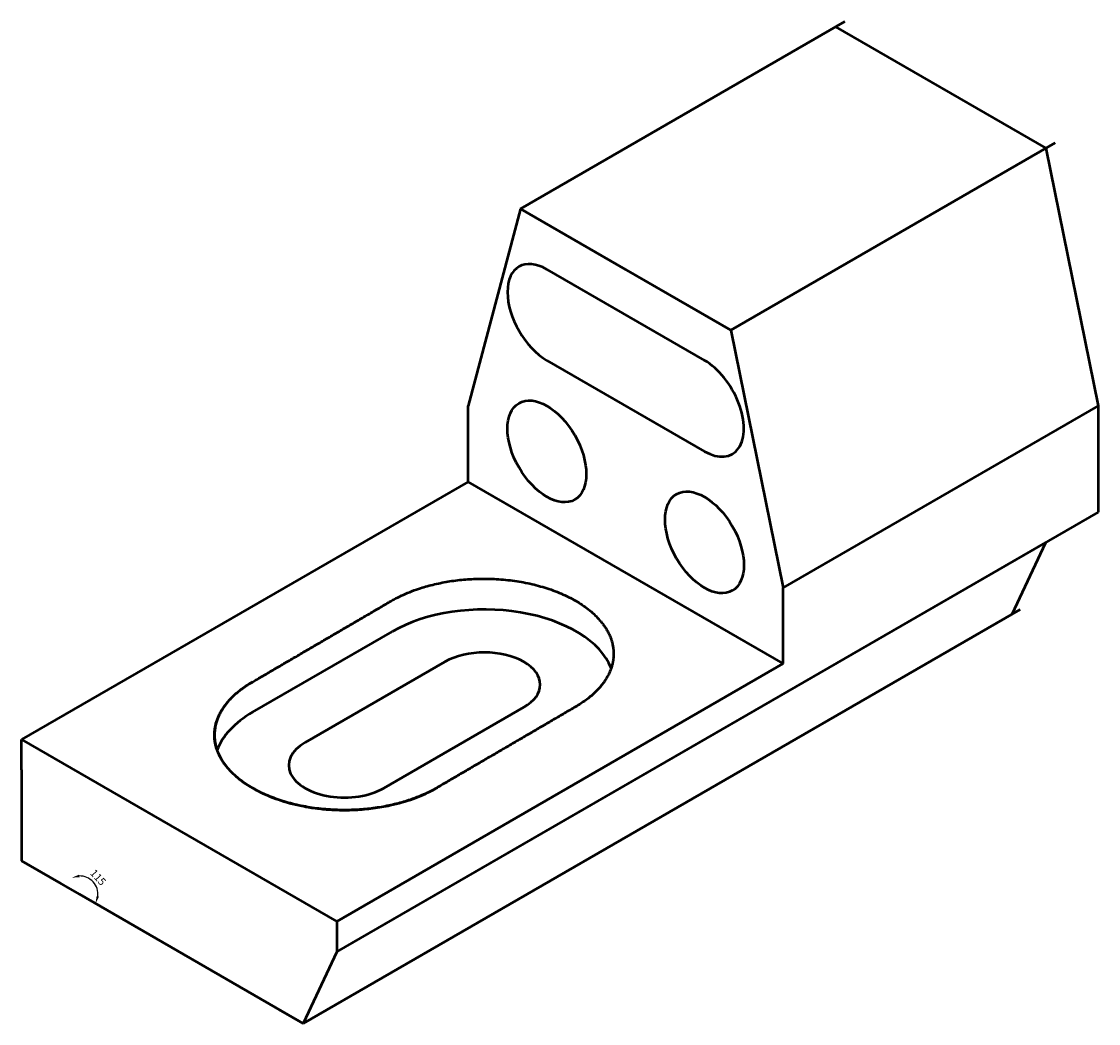
# Model space of a CAD drawing. Units: millimetres. Extents: x 15418 to 15773, y 14576 to 14907.
import ezdxf

# ---------------------------------------------------------------- set-up
doc = ezdxf.new("R2010")
doc.units = ezdxf.units.MM
doc.layers.add('M-DIMS', color=2, linetype='Continuous', lineweight=25)
doc.layers.add('M-OUTL', color=7, linetype='Continuous', lineweight=50)
doc.styles.get("Standard").update_dxf_attribs({"font": 'arial.ttf'})
doc.dimstyles.new('ISO-25', dxfattribs={"dimtxt": 2.5, "dimasz": 2.5, "dimexe": 1.25, "dimexo": 0.625, "dimtad": 1, "dimtxsty": 'Standard', "dimcen": 2.5, "dimadec": 0, "dimazin": 0, "dimtfac": 1, "dimtmove": 0, "dimatfit": 3, "dimfxl": 1, "dimarcsym": 0})

# ---------------------------------------------------------------- blocks, each defined once
blk = doc.blocks.new('*D1')
at = {"layer": 'Defpoints', "color": 0, "transparency": 16777216}
for p in [(15417.64, 14659.84), (15436.79, 14618.79), (15436.79, 14618.79), (15442.53, 14620.7), (15510.54, 14576.21)]:
    blk.add_point(p, dxfattribs=at)
at = {"layer": 'M-DIMS', "color": 0, "lineweight": -2, "transparency": 16777216}
blk.add_arc((15436.79, 14618.79), 6.05, 353.8367, 91.1633, dxfattribs=at)
at = {"layer": 'M-DIMS', "color": 0, "transparency": 16777216}
for points in [[(15436.76, 14624.44), (15436.57, 14625.25), (15434.23, 14624.28)], [(15443.2, 14618.01), (15442.41, 14618.27), (15442.03, 14615.77)]]:
    blk.add_solid(points, dxfattribs=at)
at = {"layer": 'M-DIMS', "color": 0, "transparency": 16777216, "insert": (15442.65, 14624.17), "char_height": 2.5, "attachment_point": 5, "rotation": 312.5}
blk.add_mtext('115', dxfattribs=at)

msp = doc.modelspace()

# ---------------------------------------------------------------- linework, layer by layer
at = {"layer": 'M-OUTL'}
for p, q in [((15582.188, 14844.845), (15689.103, 14906.572)), ((15686.028, 14904.845), (15755.31, 14864.845)), ((15651.47, 14804.845), (15758.385, 14866.572)), ((15755.31, 14864.845), (15772.631, 14779.845)), ((15582.188, 14844.845), (15564.867, 14779.845)), ((15651.47, 14804.845), (15582.188, 14844.845)), ((15616.829, 14824.845), (15582.188, 14844.845)), ((15590.848, 14824.845), (15642.81, 14794.845)), ((15616.829, 14824.845), (15651.47, 14804.845)), ((15616.829, 14824.845), (15651.47, 14804.845)), ((15651.47, 14804.845), (15668.79, 14719.845)), ((15590.848, 14794.845), (15642.81, 14764.845)), ((15564.867, 14754.845), (15564.867, 14779.845)), ((15668.79, 14719.845), (15772.713, 14779.845)), ((15772.713, 14744.845), (15772.713, 14779.845)), ((15564.867, 14754.845), (15417.643, 14669.845)), ((15668.79, 14694.845), (15564.867, 14754.845)), ((15521.566, 14599.845), (15772.713, 14744.845)), ((15521.566, 14599.845), (15755.393, 14734.845)), ((15521.566, 14599.845), (15755.393, 14734.845)), ((15744.288, 14711.209), (15755.31, 14734.845)), ((15668.79, 14694.845), (15668.79, 14719.845)), ((15510.544, 14576.208), (15746.881, 14712.657)), ((15493.804, 14678.816), (15539.929, 14705.446)), ((15511.125, 14668.816), (15557.25, 14695.446)), ((15521.566, 14609.845), (15668.79, 14694.845)), ((15521.566, 14609.845), (15668.79, 14694.845)), ((15537.106, 14653.816), (15583.23, 14680.446)), ((15600.285, 14680.6), (15600.285, 14680.6)), ((15417.643, 14659.845), (15417.643, 14669.845)), ((15417.643, 14669.845), (15521.566, 14609.845)), ((15417.643, 14659.845), (15417.643, 14629.845)), ((15436.786, 14618.792), (15417.643, 14629.845)), ((15417.643, 14629.845), (15430.633, 14622.345)), ((15436.786, 14618.792), (15510.544, 14576.208)), ((15521.566, 14609.845), (15521.566, 14599.845)), ((15521.566, 14609.845), (15521.566, 14599.845)), ((15521.566, 14609.845), (15521.566, 14599.845)), ((15521.566, 14599.845), (15510.544, 14576.208)), ((15510.544, 14576.208), (15502.514, 14580.845)), ((15510.544, 14576.208), (15508.576, 14577.345))]:
    msp.add_line(p, q, dxfattribs=at)
for centre, major_axis, start_param, end_param in [((15590.848, 14809.845), (9.186, -15.91), 2.3561945, 5.4977871), ((15642.81, 14779.845), (9.186, -15.91), 5.4977871, 8.6393798), ((15570.24, 14687.946), (-42.866, 0), 3.3633519, 5.4977871), ((15570.24, 14687.946), (-18.371, 0), 2.3561945, 5.4977871), ((15524.115, 14661.316), (-42.866, 0), 5.4977871, 6.079757), ((15524.115, 14661.316), (-18.371, 0), 5.4977871, 8.6393798)]:
    msp.add_ellipse(centre, major_axis=major_axis, ratio=0.5773503, start_param=start_param, end_param=end_param, dxfattribs=at)
for centre in [(15590.848, 14764.845), (15642.81, 14734.845)]:
    msp.add_ellipse(centre, major_axis=(9.186, -15.91), ratio=0.5773503, dxfattribs=at)
msp.add_rational_spline([(15600.285, 14680.6), (15617.824, 14690.726), (15611.358, 14704.552), (15604.892, 14718.377), (15580.909, 14722.03), (15556.925, 14725.683), (15539.488, 14715.499), (15516.646, 14702.157), (15493.804, 14688.816), (15476.227, 14678.668), (15482.753, 14664.819), (15489.279, 14650.97), (15513.339, 14647.362), (15537.399, 14643.754), (15554.773, 14654.019), (15577.529, 14667.31), (15600.285, 14680.6)], [1, 0.865543206449, 1, 0.865543206449, 1, 0.865543206449, 1, 1, 1, 0.865063864722, 1, 0.865063864722, 1, 0.865063864722, 1, 1, 1], degree=2, knots=[0, 0, 0, 1.0491247, 1.0491247, 2.0982495, 2.0982495, 3.1473742, 3.1473742, 4.1473742, 4.1473742, 5.1984115, 5.1984115, 6.2494488, 6.2494488, 7.3004862, 7.3004862, 8.3004862, 8.3004862, 8.3004862], dxfattribs=at)
msp.add_open_spline([(15493.804, 14688.816), (15492.652, 14688.151), (15491.557, 14687.443), (15489.983, 14686.297), (15489.463, 14685.893), (15488.467, 14685.069), (15487.991, 14684.648), (15487.14, 14683.845), (15486.762, 14683.465), (15485.359, 14681.966), (15484.481, 14680.829), (15483.462, 14679.18), (15483.212, 14678.734), (15482.75, 14677.825), (15482.541, 14677.364), (15482.196, 14676.506), (15482.055, 14676.109), (15481.846, 14675.441), (15481.772, 14675.179), (15481.634, 14674.637), (15481.572, 14674.361), (15481.402, 14673.49), (15481.323, 14672.884), (15481.266, 14672.058), (15481.256, 14671.818), (15481.245, 14671.218), (15481.252, 14670.841), (15481.298, 14670.07), (15481.337, 14669.679), (15481.44, 14668.954), (15481.501, 14668.618), (15481.605, 14668.13), (15481.642, 14667.971), (15481.758, 14667.502), (15481.848, 14667.181), (15482.05, 14666.545), (15482.161, 14666.229), (15482.524, 14665.292), (15482.802, 14664.686), (15483.368, 14663.617), (15483.635, 14663.16), (15484.702, 14661.501), (15485.657, 14660.304), (15487.441, 14658.481), (15488.147, 14657.831), (15489.721, 14656.523), (15490.599, 14655.866), (15492.454, 14654.613), (15493.435, 14654.013), (15495.854, 14652.675), (15497.318, 14651.969), (15499.977, 14650.849), (15501.143, 14650.407), (15503.519, 14649.597), (15504.733, 14649.228), (15507.311, 14648.533), (15508.673, 14648.214), (15510.958, 14647.756), (15511.877, 14647.591), (15513.583, 14647.322), (15514.369, 14647.211), (15515.973, 14647.014), (15516.785, 14646.927), (15519.249, 14646.709), (15520.925, 14646.617), (15524.323, 14646.549), (15526.036, 14646.573), (15529.699, 14646.753), (15531.654, 14646.927), (15535.498, 14647.43), (15537.39, 14647.757), (15540.562, 14648.447), (15541.862, 14648.774), (15544.381, 14649.494), (15545.603, 14649.887), (15547.913, 14650.717), (15549.006, 14651.153), (15551.091, 14652.068), (15552.085, 14652.548), (15553.632, 14653.363), (15554.212, 14653.687), (15554.773, 14654.019)], degree=3, knots=[4.1473742, 4.1473742, 4.1473742, 4.1473742, 4.2665043, 4.2665043, 4.3278748, 4.3278748, 4.3892452, 4.3892452, 4.4420419, 4.4420419, 4.5921938, 4.5921938, 4.6482961, 4.6482961, 4.7043985, 4.7043985, 4.7522672, 4.7522672, 4.7852264, 4.7852264, 4.8181856, 4.8181856, 4.8879653, 4.8879653, 4.9172569, 4.9172569, 4.9634806, 4.9634806, 5.0097044, 5.0097044, 5.0504344, 5.0504344, 5.0705038, 5.0705038, 5.1106427, 5.1106427, 5.1507816, 5.1507816, 5.2310594, 5.2310594, 5.291238, 5.291238, 5.4513022, 5.4513022, 5.5437872, 5.5437872, 5.6416988, 5.6416988, 5.7396103, 5.7396103, 5.8701507, 5.8701507, 5.9659812, 5.9659812, 6.0618118, 6.0618118, 6.1661168, 6.1661168, 6.2357701, 6.2357701, 6.2951926, 6.2951926, 6.3546151, 6.3546151, 6.4734601, 6.4734601, 6.592305, 6.592305, 6.7271887, 6.7271887, 6.8620724, 6.8620724, 6.959111, 6.959111, 7.0561496, 7.0561496, 7.1489864, 7.1489864, 7.2418231, 7.2418231, 7.3004862, 7.3004862, 7.3004862, 7.3004862], dxfattribs=at)

# ---------------------------------------------------------------- dimensions: what is measured, and where the dimension line sits
at = {"layer": 'M-DIMS'}
dim = msp.add_angular_dim_2l(base=(15442.532, 14620.696), line1=((15436.786, 14618.792), (15510.544, 14576.208)), line2=((15436.786, 14618.792), (15417.643, 14659.845)), text='115', dimstyle='ISO-25', override={"dimclrd": 0, "dimclre": 0, "dimclrt": 0}, dxfattribs=at)
dim.commit()
dim.dimension.update_dxf_attribs({"geometry": '*D1', "text_midpoint": (15442.65, 14624.166)})

doc.saveas('drawing.dxf')
